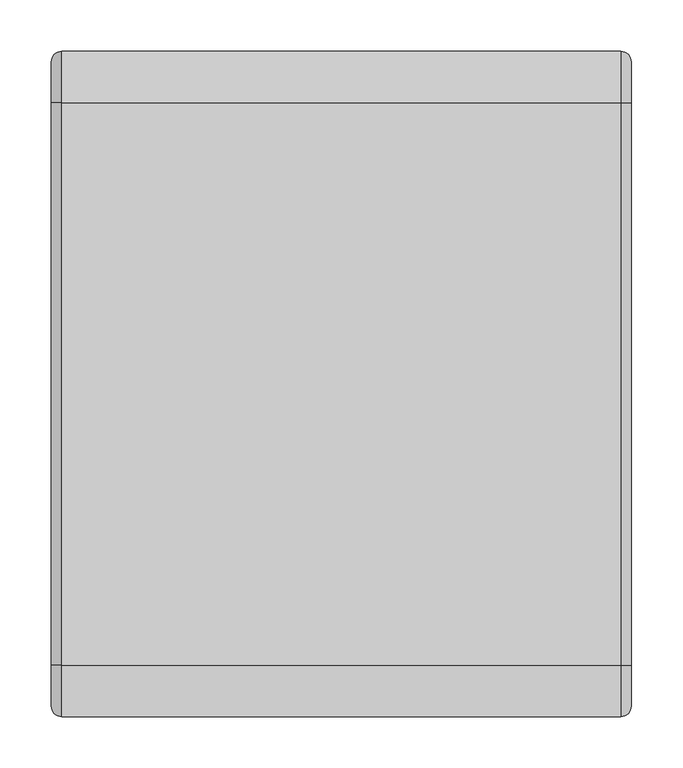
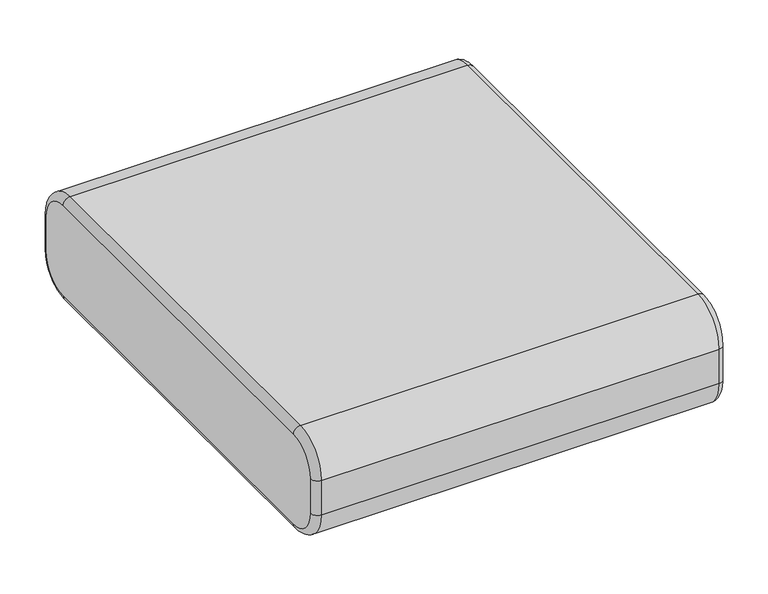
"""IFC4 building model written with IfcOpenShell, lengths in millimetres: furniture geometry."""

from ifc_helpers import new_model, si_unit, point, frame, origin, place, context, project, spatial, circle_curve, ellipse_curve, trimmed, source, transform, mapped, element, save
from ifc_brep_helpers import plane_surface, cylinder_surface, revolved_surface, advanced_brep


def furniture_402a1f5e(model_context):
    return source(origin(), model_context, "Body", "AdvancedBrep", [
        advanced_brep(
        [(282.5, 547.7044583, 315.0), (282.5, 587.7044583, 355.0), (282.5, 587.7044583, 405.0), (282.5, 547.7044583, 445.0), (282.5, 0.0, 445.0), (282.5, -40.0, 405.0), (282.5, -40.0, 355.0), (282.5, 0.0, 315.0), (-282.5, 0.0, 315.0), (-282.5, -40.0, 355.0), (-282.5, -40.0, 405.0), (-282.5, 0.0, 445.0), (-282.5, 547.7044583, 445.0), (-282.5, 587.7044583, 405.0), (-282.5, 587.7044583, 355.0), (-282.5, 547.7044583, 315.0), (-272.5, 597.7044583, 405.0), (-272.5, 547.7044583, 455.0), (272.5000135, 547.7044583, 455.0), (272.5, 597.7044583, 405.0), (-272.5, 0.0, 455.0), (272.5, 0.0, 455.0), (-272.5, -50.0, 405.0), (272.5000135, -50.0, 405.0), (-272.5, -50.0, 355.0), (272.5, -50.0, 355.0), (-272.5, 0.0, 305.0), (272.5000135, 0.0, 305.0), (-272.5, 547.7044583, 305.0), (272.5000135, 547.7044583, 305.0), (-272.5, 597.7044583, 355.0), (272.5000135, 597.7044583, 355.0)],
        [
            (0, 1, circle_curve(frame((282.5, 547.7044583, 355.0), z_axis=(1.0, 0.0, 0.0), x_axis=(0.0, 0.0, -1.0)), 40.0)),
            (1, 2),
            (2, 3, circle_curve(frame((282.5, 547.7044583, 405.0), z_axis=(1.0, 0.0, 0.0), x_axis=(0.0, 1.0, 0.0)), 40.0)),
            (3, 4),
            (4, 5, circle_curve(frame((282.5, 0.0, 405.0), z_axis=(1.0, 0.0, 0.0), x_axis=(0.0, 0.0, 1.0)), 40.0)),
            (5, 6),
            (6, 7, circle_curve(frame((282.5, 0.0, 355.0), z_axis=(1.0, 0.0, 0.0), x_axis=(0.0, -1.0, 0.0)), 40.0)),
            (7, 0),
            (8, 9, circle_curve(frame((-282.5, 0.0, 355.0), z_axis=(-1.0, 0.0, 0.0), x_axis=(0.0, 0.0, -1.0)), 40.0)),
            (9, 10),
            (10, 11, circle_curve(frame((-282.5, 0.0, 405.0), z_axis=(-1.0, 0.0, 0.0), x_axis=(0.0, -1.0, 0.0)), 40.0)),
            (11, 12),
            (12, 13, circle_curve(frame((-282.5, 547.7044583, 405.0), z_axis=(-1.0, 0.0, 0.0), x_axis=(0.0, 0.0, 1.0)), 40.0)),
            (13, 14),
            (14, 15, circle_curve(frame((-282.5, 547.7044583, 355.0), z_axis=(-1.0, 0.0, 0.0), x_axis=(0.0, 1.0, 0.0)), 40.0)),
            (15, 8),
            (16, 17, circle_curve(frame((-272.5, 547.7044583, 405.0), z_axis=(1.0, 0.0, 0.0), x_axis=(0.0, 1.0, 0.0)), 50.0)),
            (17, 18),
            (18, 19, circle_curve(frame((272.5, 547.7044583, 405.0), z_axis=(-1.0, 0.0, 0.0), x_axis=(0.0, 1.0, 0.0)), 50.0)),
            (19, 16),
            (17, 20),
            (20, 21),
            (21, 18),
            (20, 22, circle_curve(frame((-272.5, 0.0, 405.0), z_axis=(1.0, 0.0, 0.0), x_axis=(0.0, 1.0, 0.0)), 50.0)),
            (22, 23),
            (23, 21, circle_curve(frame((272.5, 0.0, 405.0), z_axis=(-1.0, 0.0, 0.0), x_axis=(0.0, 1.0, 0.0)), 50.0)),
            (22, 24),
            (24, 25),
            (25, 23),
            (24, 26, circle_curve(frame((-272.5, 0.0, 355.0), z_axis=(1.0, 0.0, 0.0), x_axis=(0.0, 1.0, 0.0)), 50.0)),
            (26, 27),
            (27, 25, circle_curve(frame((272.5, 0.0, 355.0), z_axis=(-1.0, 0.0, 0.0), x_axis=(0.0, 1.0, 0.0)), 50.0)),
            (26, 28),
            (28, 29),
            (29, 27),
            (28, 30, circle_curve(frame((-272.5, 547.7044583, 355.0), z_axis=(1.0, 0.0, 0.0), x_axis=(0.0, 1.0, 0.0)), 50.0)),
            (30, 31),
            (31, 29, circle_curve(frame((272.5, 547.7044583, 355.0), z_axis=(-1.0, 0.0, 0.0), x_axis=(0.0, 1.0, 0.0)), 50.0)),
            (30, 16),
            (19, 31),
            (24, 9, circle_curve(frame((-272.5, -40.0, 355.0), z_axis=(0.0, 0.0, -1.0), x_axis=(-1.0, 0.0, 0.0)), 10.0)),
            (8, 26, circle_curve(frame((-272.5, 0.0, 315.0), z_axis=(0.0, -1.0, 0.0), x_axis=(-1.0, 0.0, 0.0)), 10.0)),
            (22, 10, circle_curve(frame((-272.5, -40.0, 405.0), z_axis=(0.0, 0.0, -1.0), x_axis=(-1.0, 0.0, 0.0)), 10.0)),
            (20, 11, circle_curve(frame((-272.5, 0.0, 445.0), z_axis=(0.0, -1.0, 0.0), x_axis=(-1.0, 0.0, 0.0)), 10.0)),
            (17, 12, circle_curve(frame((-272.5, 547.7044583, 445.0), z_axis=(0.0, -1.0, 0.0), x_axis=(-1.0, 0.0, 0.0)), 10.0)),
            (16, 13, circle_curve(frame((-272.5, 587.7044583, 405.0), z_axis=(0.0, 0.0, 1.0), x_axis=(-1.0, 0.0, 0.0)), 10.0)),
            (30, 14, circle_curve(frame((-272.5, 587.7044583, 355.0), z_axis=(0.0, 0.0, 1.0), x_axis=(-1.0, 0.0, 0.0)), 10.0)),
            (28, 15, circle_curve(frame((-272.5, 547.7044583, 315.0), z_axis=(0.0, 1.0, 0.0), x_axis=(-1.0, 0.0, 0.0)), 10.0)),
            (31, 1, circle_curve(frame((272.5, 587.7044583, 355.0), z_axis=(0.0, 0.0, -1.0), x_axis=(1.0, 0.0, 0.0)), 10.0)),
            (0, 29, circle_curve(frame((272.5, 547.7044583, 315.0), z_axis=(0.0, 1.0, 0.0), x_axis=(1.0, 0.0, 0.0)), 10.0)),
            (19, 2, circle_curve(frame((272.5, 587.7044583, 405.0), z_axis=(0.0, 0.0, -1.0), x_axis=(1.0, 0.0, 0.0)), 10.0)),
            (18, 3, circle_curve(frame((272.5, 547.7044583, 445.0), z_axis=(0.0, 1.0, 0.0), x_axis=(1.0, 0.0, 0.0)), 10.0)),
            (21, 4, circle_curve(frame((272.5, 0.0, 445.0), z_axis=(0.0, 1.0, 0.0), x_axis=(1.0, 0.0, 0.0)), 10.0)),
            (23, 5, circle_curve(frame((272.5, -40.0, 405.0), z_axis=(0.0, 0.0, 1.0), x_axis=(1.0, 0.0, 0.0)), 10.0)),
            (25, 6, circle_curve(frame((272.5, -40.0, 355.0), z_axis=(0.0, 0.0, 1.0), x_axis=(1.0, 0.0, 0.0)), 10.0)),
            (27, 7, circle_curve(frame((272.5, 0.0, 315.0), z_axis=(0.0, -1.0, 0.0), x_axis=(1.0, 0.0, 0.0)), 10.0)),
        ],
        [
            plane_surface(frame((282.5, 597.7044583, 405.0), z_axis=(1.0, 0.0, 0.0), x_axis=(0.0, 0.0, 1.0))),
            plane_surface(frame((-282.5, 597.7044583, 405.0), z_axis=(-1.0, 0.0, 0.0), x_axis=(0.0, 0.0, -1.0))),
            cylinder_surface(frame((-282.5, 547.7044583, 405.0), z_axis=(1.0, 0.0, 0.0), x_axis=(0.0, 1.0, 0.0)), 50.0),
            plane_surface(frame((282.5, 547.7044583, 455.0), z_axis=(0.0, 0.0, 1.0), x_axis=(-1.0, 0.0, 0.0))),
            cylinder_surface(frame((-282.5, 0.0, 405.0), z_axis=(1.0, 0.0, 0.0), x_axis=(0.0, 1.0, 0.0)), 50.0),
            plane_surface(frame((282.5, -50.0, 405.0), z_axis=(0.0, -1.0, 0.0), x_axis=(-1.0, 0.0, 0.0))),
            cylinder_surface(frame((-282.5, 0.0, 355.0), z_axis=(1.0, 0.0, 0.0), x_axis=(0.0, 1.0, 0.0)), 50.0),
            plane_surface(frame((282.5, 0.0, 305.0), z_axis=(0.0, 0.0, -1.0), x_axis=(-1.0, 0.0, 0.0))),
            cylinder_surface(frame((-282.5, 547.7044583, 355.0), z_axis=(1.0, 0.0, 0.0), x_axis=(0.0, 1.0, 0.0)), 50.0),
            plane_surface(frame((282.5, 597.7044583, 355.0), z_axis=(0.0, 1.0, 0.0), x_axis=(-1.0, 0.0, 0.0))),
            revolved_surface(trimmed(ellipse_curve(frame((-272.5, 0.0, 315.0), z_axis=(0.0, 1.0, 0.0), x_axis=(-1.0, 0.0, 0.0)), 10.0, 10.0), [point((-272.5, 0.0, 305.0))], [point((-282.5, 0.0, 315.0))], True, "CARTESIAN"), (-282.5, 0.0, 355.0), (-1.0, 0.0, 0.0)),
            cylinder_surface(frame((-272.5, -40.0, 355.0), z_axis=(0.0, 0.0, 1.0), x_axis=(-1.0, 0.0, 0.0)), 10.0),
            revolved_surface(trimmed(ellipse_curve(frame((-272.5, -40.0, 405.0), z_axis=(0.0, 0.0, -1.0), x_axis=(-1.0, 0.0, 0.0)), 10.0, 10.0), [point((-272.5, -50.0, 405.0))], [point((-282.5, -40.0, 405.0))], True, "CARTESIAN"), (-282.5, 0.0, 405.0), (-1.0, 0.0, 0.0)),
            cylinder_surface(frame((-272.5, 0.0, 445.0), z_axis=(0.0, 1.0, 0.0), x_axis=(-1.0, 0.0, 0.0)), 10.0),
            revolved_surface(trimmed(ellipse_curve(frame((-272.5, 547.7044583, 445.0), z_axis=(0.0, -1.0, 0.0), x_axis=(-1.0, 0.0, 0.0)), 10.0, 10.0), [point((-272.5, 547.7044583, 455.0))], [point((-282.5, 547.7044583, 445.0))], True, "CARTESIAN"), (-282.5, 547.7044583, 405.0), (-1.0, 0.0, 0.0)),
            cylinder_surface(frame((-272.5, 587.7044583, 405.0), z_axis=(0.0, 0.0, -1.0), x_axis=(-1.0, 0.0, 0.0)), 10.0),
            revolved_surface(trimmed(ellipse_curve(frame((-272.5, 587.7044583, 355.0), z_axis=(0.0, 0.0, 1.0), x_axis=(-1.0, 0.0, 0.0)), 10.0, 10.0), [point((-272.5, 597.7044583, 355.0))], [point((-282.5, 587.7044583, 355.0))], True, "CARTESIAN"), (-282.5, 547.7044583, 355.0), (-1.0, 0.0, 0.0)),
            cylinder_surface(frame((-272.5, 547.7044583, 315.0), z_axis=(0.0, -1.0, 0.0), x_axis=(-1.0, 0.0, 0.0)), 10.0),
            revolved_surface(trimmed(ellipse_curve(frame((272.5, 547.7044583, 315.0), z_axis=(0.0, -1.0, 0.0), x_axis=(1.0, 0.0, 0.0)), 10.0, 10.0), [point((272.5, 547.7044583, 305.0))], [point((282.5, 547.7044583, 315.0))], True, "CARTESIAN"), (282.5, 547.7044583, 355.0), (1.0, 0.0, 0.0)),
            cylinder_surface(frame((272.5, 587.7044583, 355.0), z_axis=(0.0, 0.0, 1.0), x_axis=(1.0, 0.0, 0.0)), 10.0),
            revolved_surface(trimmed(ellipse_curve(frame((272.5, 587.7044583, 405.0), z_axis=(0.0, 0.0, -1.0), x_axis=(1.0, 0.0, 0.0)), 10.0, 10.0), [point((272.5, 597.7044583, 405.0))], [point((282.5, 587.7044583, 405.0))], True, "CARTESIAN"), (282.5, 547.7044583, 405.0), (1.0, 0.0, 0.0)),
            cylinder_surface(frame((272.5, 547.7044583, 445.0), z_axis=(0.0, -1.0, 0.0), x_axis=(1.0, 0.0, 0.0)), 10.0),
            revolved_surface(trimmed(ellipse_curve(frame((272.5, 0.0, 445.0), z_axis=(0.0, 1.0, 0.0), x_axis=(1.0, 0.0, 0.0)), 10.0, 10.0), [point((272.5, 0.0, 455.0))], [point((282.5, 0.0, 445.0))], True, "CARTESIAN"), (282.5, 0.0, 405.0), (1.0, 0.0, 0.0)),
            cylinder_surface(frame((272.5, -40.0, 405.0), z_axis=(0.0, 0.0, -1.0), x_axis=(1.0, 0.0, 0.0)), 10.0),
            revolved_surface(trimmed(ellipse_curve(frame((272.5, -40.0, 355.0), z_axis=(0.0, 0.0, 1.0), x_axis=(1.0, 0.0, 0.0)), 10.0, 10.0), [point((272.5, -50.0, 355.0))], [point((282.5, -40.0, 355.0))], True, "CARTESIAN"), (282.5, 0.0, 355.0), (1.0, 0.0, 0.0)),
            cylinder_surface(frame((272.5, 0.0, 315.0), z_axis=(0.0, 1.0, 0.0), x_axis=(1.0, 0.0, 0.0)), 10.0),
        ],
        [
            (0, [[1, 2, 3, 4, 5, 6, 7, 8]]),
            (1, [[9, 10, 11, 12, 13, 14, 15, 16]]),
            (2, [[17, 18, 19, 20]]),
            (3, [[21, 22, 23, -18]]),
            (4, [[24, 25, 26, -22]]),
            (5, [[27, 28, 29, -25]]),
            (6, [[30, 31, 32, -28]]),
            (7, [[33, 34, 35, -31]]),
            (8, [[36, 37, 38, -34]]),
            (9, [[39, -20, 40, -37]]),
            (10, [[41, -9, 42, -30]]),
            (11, [[-41, -27, 43, -10]]),
            (12, [[-43, -24, 44, -11]]),
            (13, [[-44, -21, 45, -12]]),
            (14, [[-45, -17, 46, -13]]),
            (15, [[-46, -39, 47, -14]]),
            (16, [[-47, -36, 48, -15]]),
            (17, [[-42, -16, -48, -33]]),
            (18, [[49, -1, 50, -38]]),
            (19, [[-49, -40, 51, -2]]),
            (20, [[-51, -19, 52, -3]]),
            (21, [[-52, -23, 53, -4]]),
            (22, [[-53, -26, 54, -5]]),
            (23, [[-54, -29, 55, -6]]),
            (24, [[-55, -32, 56, -7]]),
            (25, [[-50, -8, -56, -35]]),
        ],
    ),
    ])


if __name__ == "__main__":
    model = new_model("IFC4")
    model_context = context("Model", 3, world=origin())
    ifc_project = project(units=[si_unit("LENGTHUNIT", "METRE", prefix="MILLI")], contexts=[model_context])
    site = spatial("IfcSite", under=ifc_project)
    building = spatial("IfcBuilding", under=site)
    placement = place(None, origin())
    furniture_shape = furniture_402a1f5e(model_context)
    element("IfcFurniture", 1, at=placement, inside=building, context=model_context, shape_type="MappedRepresentation", body=[
        mapped(furniture_shape, transform((0.0, 0.0, 0.0), x_axis=(1.0, 0.0, 0.0), y_axis=(0.0, 1.0, 0.0), z_axis=(0.0, 0.0, 1.0))),
    ])
    save(model, "model.ifc")

# Revit data of these elements
# Type
#   Width [instance] = 2' - 6.31496"
#   Default Elevation = 0
